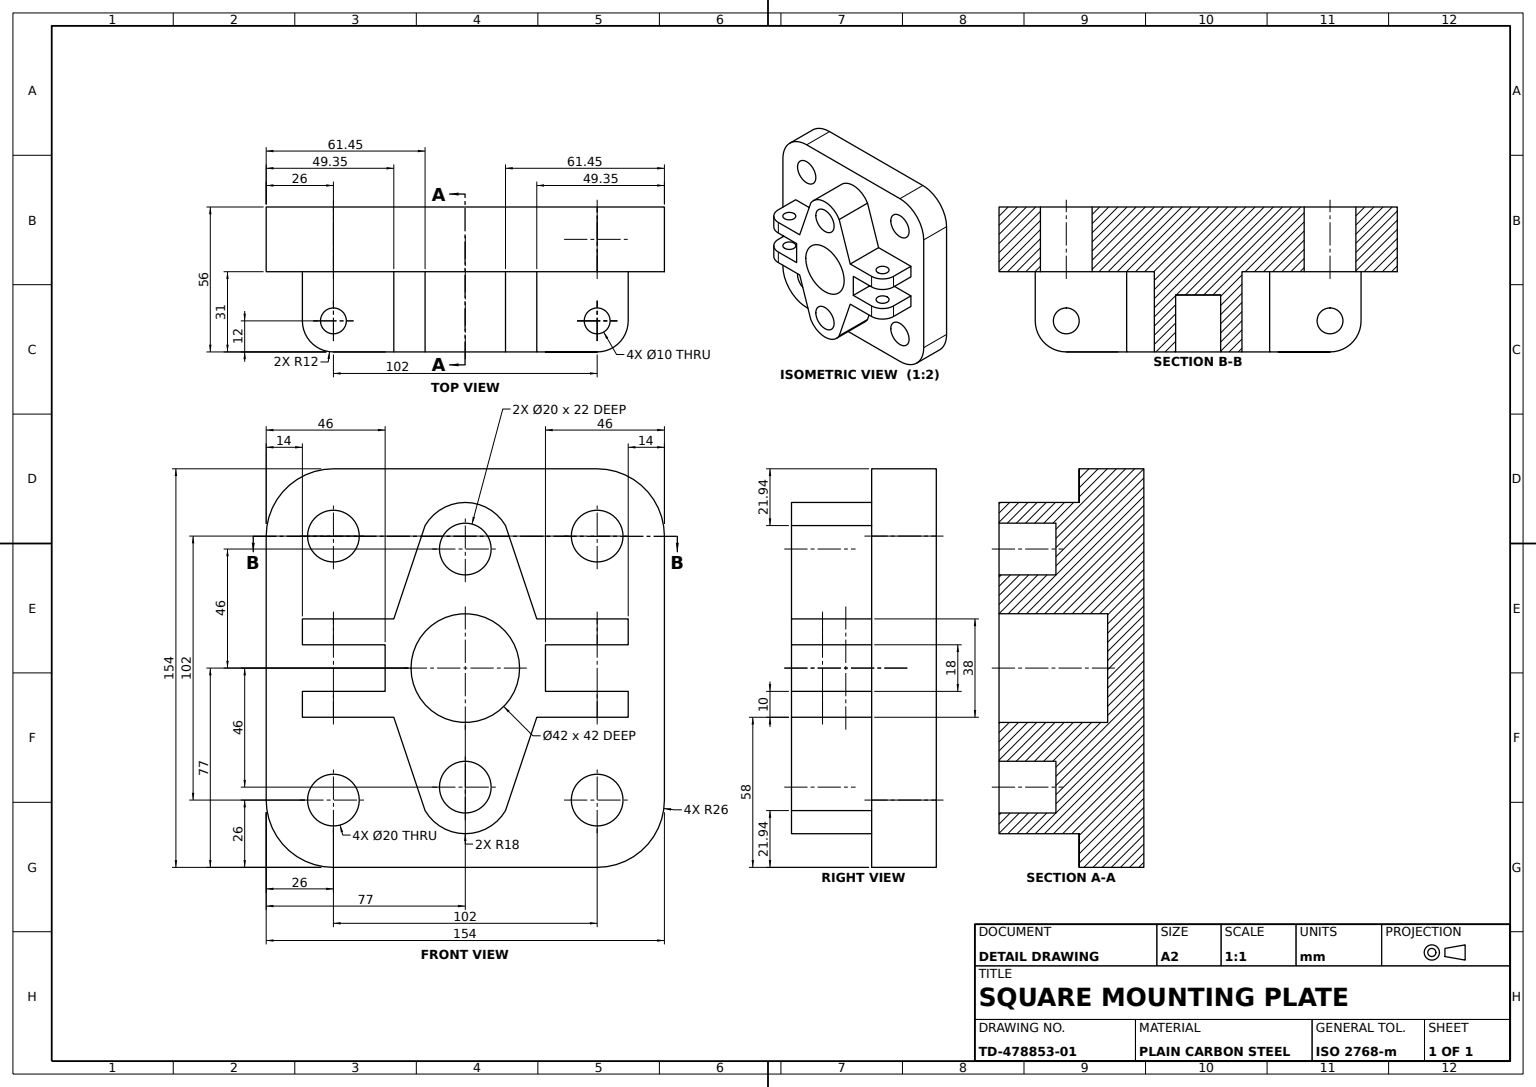
from build123d import *

# Parameters (mm, degrees)
BASE_PLATE_DEPTH         = 25
FLANGE_BOSS_DEPTH        = 31
LUG_SLOT_1_DEPTH         = 50
LUG_SLOT_2_DEPTH         = 50
LUG_PIN_HOLES_SKETCH_R   = 5
LUG_PIN_HOLES_2X_DEPTH   = 50
FLANGE_HOLES_SKETCH_R    = 10
FLANGE_HOLES_2X_DEPTH    = 22
CENTRE_BORE_SKETCH_R     = 21
CENTRE_BORE_42_DEPTH     = 42
CORNER_HOLES_SKETCH_R    = 10
CORNER_HOLES_4X_20_DEPTH = 42


with BuildPart() as part:
    # Base Plate Sketch → Base Plate (new body)
    with BuildSketch(Plane.XY):
        with BuildLine():
            Line((0, -26), (0, -128))
            ThreePointArc((0, -128), (7.615223689, -146.384776311), (26, -154))
            Line((26, -154), (128, -154))
            ThreePointArc((128, -154), (146.384776311, -146.384776311), (154, -128))
            Line((154, -128), (154, -26))
            ThreePointArc((154, -26), (146.384776311, -7.615223689), (128, 0))
            Line((128, 0), (26, 0))
            ThreePointArc((26, 0), (7.615223689, -7.615223689), (0, -26))
        make_face()
    extrude(amount=BASE_PLATE_DEPTH)

    # Flange Boss Sketch → Flange Boss (add)
    with BuildSketch(Plane.XY.offset(25)):
        with BuildLine():
            Line((14, -96), (49.353610872, -96))
            Line((49.353610872, -96), (61.447265664, -132.061592281))
            ThreePointArc((61.447265664, -132.061592281), (77, -141), (92.552734336, -132.061592281))
            Line((92.552734336, -132.061592281), (104.646389128, -96))
            Line((104.646389128, -96), (140, -96))
            Line((140, -96), (140, -86))
            Line((140, -86), (108, -86))
            Line((108, -86), (108, -68))
            Line((108, -68), (140, -68))
            Line((140, -68), (140, -58))
            Line((140, -58), (104.646389128, -58))
            Line((104.646389128, -58), (92.552734336, -21.938407719))
            ThreePointArc((92.552734336, -21.938407719), (77, -13), (61.447265664, -21.938407719))
            Line((61.447265664, -21.938407719), (49.353610872, -58))
            Line((49.353610872, -58), (14, -58))
            Line((14, -58), (14, -68))
            Line((14, -68), (46, -68))
            Line((46, -68), (46, -77))
            Line((46, -77), (46, -86))
            Line((46, -86), (14, -86))
            Line((14, -86), (14, -96))
        make_face()
    extrude(amount=FLANGE_BOSS_DEPTH)

    # Lug Slot 1 Sketch → Lug Slot 1 (cut)
    with BuildSketch(Plane.XZ.offset(96)):
        with BuildLine():
            Line((140, 56), (140, 44))
            ThreePointArc((140, 44), (136.485281374, 52.485281374), (128, 56))
            Line((128, 56), (140, 56))
        make_face()
    extrude(amount=-LUG_SLOT_1_DEPTH, mode=Mode.SUBTRACT)

    # Lug Slot 2 Sketch → Lug Slot 2 (cut)
    with BuildSketch(Plane.XZ.offset(96)):
        with BuildLine():
            Line((14, 56), (26, 56))
            ThreePointArc((26, 56), (17.514718626, 52.485281374), (14, 44))
            Line((14, 44), (14, 56))
        make_face()
    extrude(amount=-LUG_SLOT_2_DEPTH, mode=Mode.SUBTRACT)

    # Lug Pin Holes Sketch → Lug Pin Holes 2x (cut)
    with BuildSketch(Plane.XZ.offset(96)):
        with Locations(Location((128, 44, 0), (0, 0, 270))):
            Circle(LUG_PIN_HOLES_SKETCH_R)
        with Locations(Location((26, 44, 0), (0, 0, 270))):
            Circle(LUG_PIN_HOLES_SKETCH_R)
    extrude(amount=-LUG_PIN_HOLES_2X_DEPTH, mode=Mode.SUBTRACT)

    # Flange Holes Sketch → Flange Holes 2x (cut)
    with BuildSketch(Plane.XY.offset(56)):
        with Locations((77, -31)):
            Circle(FLANGE_HOLES_SKETCH_R)
        with Locations((77, -123)):
            Circle(FLANGE_HOLES_SKETCH_R)
    extrude(amount=-FLANGE_HOLES_2X_DEPTH, mode=Mode.SUBTRACT)

    # Centre Bore Sketch → Centre Bore Ø42 (cut)
    with BuildSketch(Plane.XY.offset(56)):
        with Locations((77, -77)):
            Circle(CENTRE_BORE_SKETCH_R)
    extrude(amount=-CENTRE_BORE_42_DEPTH, mode=Mode.SUBTRACT)

    # Corner Holes Sketch → Corner Holes 4xØ20 (cut)
    with BuildSketch(Plane.XY.offset(25)):
        with Locations((26, -26)):
            Circle(CORNER_HOLES_SKETCH_R)
        with Locations((128, -26)):
            Circle(CORNER_HOLES_SKETCH_R)
        with Locations((128, -128)):
            Circle(CORNER_HOLES_SKETCH_R)
        with Locations((26, -128)):
            Circle(CORNER_HOLES_SKETCH_R)
    extrude(amount=-CORNER_HOLES_4X_20_DEPTH, mode=Mode.SUBTRACT)


solid = part.part
